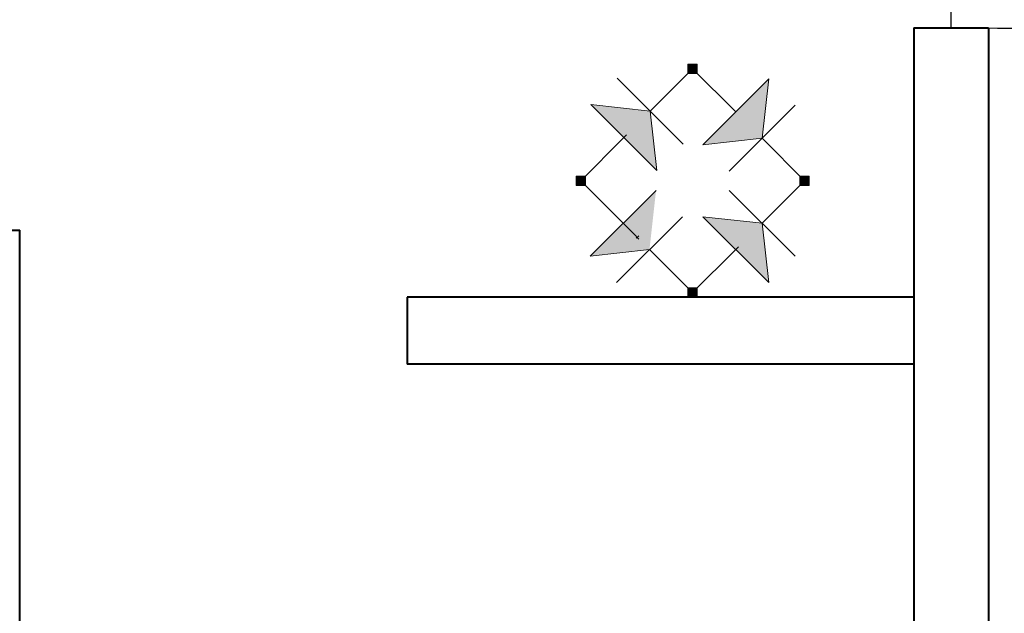
# Model space of a CAD drawing. Units: inches. Extents: x 459864 to 460310, y 324185 to 324787.
# Tile 69 of 112: x 460061 to 460127, y 324360 to 324400. Entities that reach past the tile are written whole.
import ezdxf

# ---------------------------------------------------------------- set-up
doc = ezdxf.new("R2010")
doc.units = ezdxf.units.IN
for name, color, linetype, lineweight in [('A-ANNO-DIMS', 2, 'Continuous', 18), ('A-DOOR', 3, 'Continuous', 25), ('A-FURN', 8, 'Continuous', 18), ('A-WALL', 7, 'Continuous', 40)]:
    doc.layers.add(name, color=color, linetype=linetype, lineweight=lineweight)
doc.styles.get("Standard").update_dxf_attribs({"font": 'arial.ttf'})
doc.dimstyles.new('ISO-25', dxfattribs={"dimtxt": 6, "dimasz": 2.5, "dimexe": 1.25, "dimexo": 0.625, "dimtad": 1, "dimdec": 1, "dimlunit": 3, "dimtxsty": 'Standard', "dimcen": 2.5, "dimadec": 0, "dimazin": 0, "dimtfac": 1, "dimtdec": 1, "dimtmove": 0, "dimatfit": 3, "dimfxl": 1, "dimarcsym": 0})

# ---------------------------------------------------------------- blocks, each defined once
blk = doc.blocks.new('Full Wave Bridge')
for p, q in [((0.185922, 0.186729), (0.3, 0.3)), ((0.415786, 0.185084), (0.3, 0.3)), ((0.274311, 0.098341), (0.097534, 0.275118)), ((0.327398, 0.096696), (0.504174, 0.273472)), ((0.504174, 0.273472), (0.486497, 0.114373)), ((0.026823, 0.204407), (0.185922, 0.186729)), ((0.2036, 0.02763), (0.026823, 0.204407)), ((0.185922, 0.186729), (0.2036, 0.02763)), ((0.398109, 0.025985), (0.574885, 0.202762)), ((0.115212, 0.116019), (0, 0)), ((0.115212, 0.116019), (0.122283, 0.12309)), ((0.486497, 0.114373), (0.327398, 0.096696)), ((0.486497, 0.114373), (0.6, 0)), ((0.113504, -0.114373), (0, 0)), ((0.486497, -0.114373), (0.6, 0)), ((0.025116, -0.202762), (0.201892, -0.025985)), ((0.574885, -0.202762), (0.398108, -0.025985)), ((0.095826, -0.273472), (0.272603, -0.096695)), ((0.327398, -0.096695), (0.486497, -0.114373)), ((0.504174, -0.273472), (0.327398, -0.096695)), ((0.113504, -0.114373), (0.120575, -0.121444)), ((0.120575, -0.121444), (0.127646, -0.128515)), ((0.127646, -0.128515), (0.134717, -0.135586)), ((0.486497, -0.114373), (0.504174, -0.273472)), ((0.134717, -0.135586), (0.141788, -0.142657)), ((0.141788, -0.142657), (0.15593, -0.1568)), ((0.155993, -0.148218), (0.148824, -0.154349)), ((0.415786, -0.185084), (0.422857, -0.178013)), ((0.184215, -0.185084), (0.025116, -0.202762)), ((0.184215, -0.185084), (0.3, -0.3)), ((0.415786, -0.185084), (0.3, -0.3))]:
    blk.add_line(p, q)
for points in [[(0.2875, 0.2875), (0.2875, 0.3125), (0.3125, 0.3125), (0.3125, 0.2875)], [(-0.0125, -0.0125), (-0.0125, 0.0125), (0.012501, 0.0125), (0.012501, -0.0125)], [(0.5875, -0.0125), (0.5875, 0.0125), (0.6125, 0.0125), (0.6125, -0.0125)], [(0.2875, -0.3125), (0.2875, -0.2875), (0.3125, -0.2875), (0.3125, -0.3125)]]:
    blk.add_lwpolyline(points, close=True)
for points in [[(0.3125, 0.2875), (0.3125, 0.3125), (0.2875, 0.3125)], [(0.2875, 0.3125), (0.2875, 0.2875), (0.3125, 0.2875)], [(0.327398, 0.096696), (0.486497, 0.114373), (0.504174, 0.273472)], [(0.2036, 0.02763), (0.185922, 0.186729), (0.026823, 0.204407)], [(0.012501, -0.0125), (0.012501, 0.0125), (-0.0125, 0.0125)], [(-0.0125, 0.0125), (-0.0125, -0.0125), (0.012501, -0.0125)], [(0.6125, -0.0125), (0.6125, 0.0125), (0.5875, 0.0125)], [(0.5875, 0.0125), (0.5875, -0.0125), (0.6125, -0.0125)], [(0.025116, -0.202762), (0.184215, -0.185084), (0.201892, -0.025985)], [(0.327398, -0.096695), (0.486497, -0.114373), (0.504174, -0.273472)], [(0.3125, -0.3125), (0.3125, -0.2875), (0.2875, -0.2875)], [(0.2875, -0.2875), (0.2875, -0.3125), (0.3125, -0.3125)]]:
    blk.add_solid(points)
blk = doc.blocks.new('*D28')
at = {"layer": 'A-ANNO-DIMS', "color": 0, "lineweight": -2, "transparency": 16777216}
for p, q in [((460148.65, 324370.7), (460136.025, 324370.7)), ((460137.275, 324368.2), (460137.275, 324293.2)), ((460148.65, 324290.7), (460136.025, 324290.7)), ((460137.275, 324290.7), (460137.275, 324198.69))]:
    blk.add_line(p, q, dxfattribs=at)
at = {"layer": 'A-ANNO-DIMS', "color": 0, "transparency": 16777216}
for points in [[(460136.858, 324368.2), (460137.692, 324368.2), (460137.275, 324370.7)], [(460136.858, 324293.2), (460137.692, 324293.2), (460137.275, 324290.7)]]:
    blk.add_solid(points, dxfattribs=at)
at = {"layer": 'Defpoints', "color": 0, "transparency": 16777216}
for p in [(460149.275, 324370.7), (460137.275, 324290.7), (460149.275, 324290.7)]:
    blk.add_point(p, dxfattribs=at)
at = {"layer": 'A-ANNO-DIMS', "color": 0, "transparency": 16777216, "insert": (460133.363, 324243.445), "char_height": 6, "attachment_point": 5, "rotation": 90}
blk.add_mtext('QUEEN BED 6\'-8" TYP.', dxfattribs=at)
blk = doc.blocks.new('*D69')
at = {"layer": 'A-ANNO-DIMS', "color": 0, "lineweight": -2, "transparency": 16777216}
for p, q in [((460055.99, 324376.483), (459874.965, 324376.483)), ((459876.215, 324373.983), (459876.215, 324285.983)), ((460060.49, 324283.483), (459874.965, 324283.483))]:
    blk.add_line(p, q, dxfattribs=at)
at = {"layer": 'A-ANNO-DIMS', "color": 0, "transparency": 16777216}
for points in [[(459875.798, 324373.983), (459876.632, 324373.983), (459876.215, 324376.483)], [(459875.798, 324285.983), (459876.632, 324285.983), (459876.215, 324283.483)]]:
    blk.add_solid(points, dxfattribs=at)
at = {"layer": 'Defpoints', "color": 0, "transparency": 16777216}
for p in [(460056.615, 324376.483), (459876.215, 324283.483), (460061.115, 324283.483)]:
    blk.add_point(p, dxfattribs=at)
at = {"layer": 'A-ANNO-DIMS', "color": 0, "transparency": 16777216, "insert": (459872.526, 324329.983), "char_height": 6, "attachment_point": 5, "rotation": 90}
blk.add_mtext('7\'-9"', dxfattribs=at)

msp = doc.modelspace()

# ---------------------------------------------------------------- linework, layer by layer
at = {"layer": 'A-DOOR'}
msp.add_line((460123.615, 324399.05), (460123.615, 324421.05), dxfattribs=at)
msp.add_arc((460127.115, 324422.05), 23.022, 267.51045, 2.48955, dxfattribs=at)
at = {"layer": 'A-WALL'}
for p, q in [((460121.115, 324399.05), (460126.115, 324399.05)), ((460121.115, 324399.05), (460121.115, 324283.483)), ((460126.115, 324399.05), (460126.115, 324283.483)), ((460060.068, 324385.483), (460061.115, 324385.483)), ((460061.115, 324380.983), (460061.115, 324385.483)), ((460061.115, 324323.126), (460061.115, 324380.983)), ((460121.115, 324380.983), (460087.115, 324380.983)), ((460087.115, 324380.983), (460087.115, 324376.483)), ((460121.115, 324376.483), (460087.115, 324376.483))]:
    msp.add_line(p, q, dxfattribs=at)

# ---------------------------------------------------------------- block references
at = {"layer": 'A-FURN', "xscale": 25, "yscale": 25}
msp.add_blockref('Full Wave Bridge', (460098.767, 324388.796), dxfattribs=at)

# ---------------------------------------------------------------- dimensions: what is measured, and where the dimension line sits
at = {"layer": 'A-ANNO-DIMS'}
dim = msp.add_linear_dim(base=(459876.215, 324283.483), p1=(460056.615, 324376.483), p2=(460061.115, 324283.483), angle=90, dimstyle='ISO-25', override={"dimdec": 1, "dimlfac": 1, "dimrnd": 0, "dimzin": 1, "dimdsep": 46, "dimlunit": 4, "dimfrac": 2}, dxfattribs=at)
dim.commit()
dim.dimension.update_dxf_attribs({"geometry": '*D69', "text_midpoint": (459872.526, 324329.983)})
dim = msp.add_linear_dim(base=(460137.275, 324290.7), p1=(460149.275, 324370.7), p2=(460149.275, 324290.7), angle=270, text='QUEEN BED <> TYP.', dimstyle='ISO-25', override={"dimdec": 1, "dimlfac": 1, "dimrnd": 0, "dimzin": 1, "dimdsep": 46, "dimlunit": 4, "dimfrac": 2}, dxfattribs=at)
dim.commit()
dim.dimension.update_dxf_attribs({"geometry": '*D28', "text_midpoint": (460133.363, 324243.445)})

doc.saveas('drawing.dxf')
